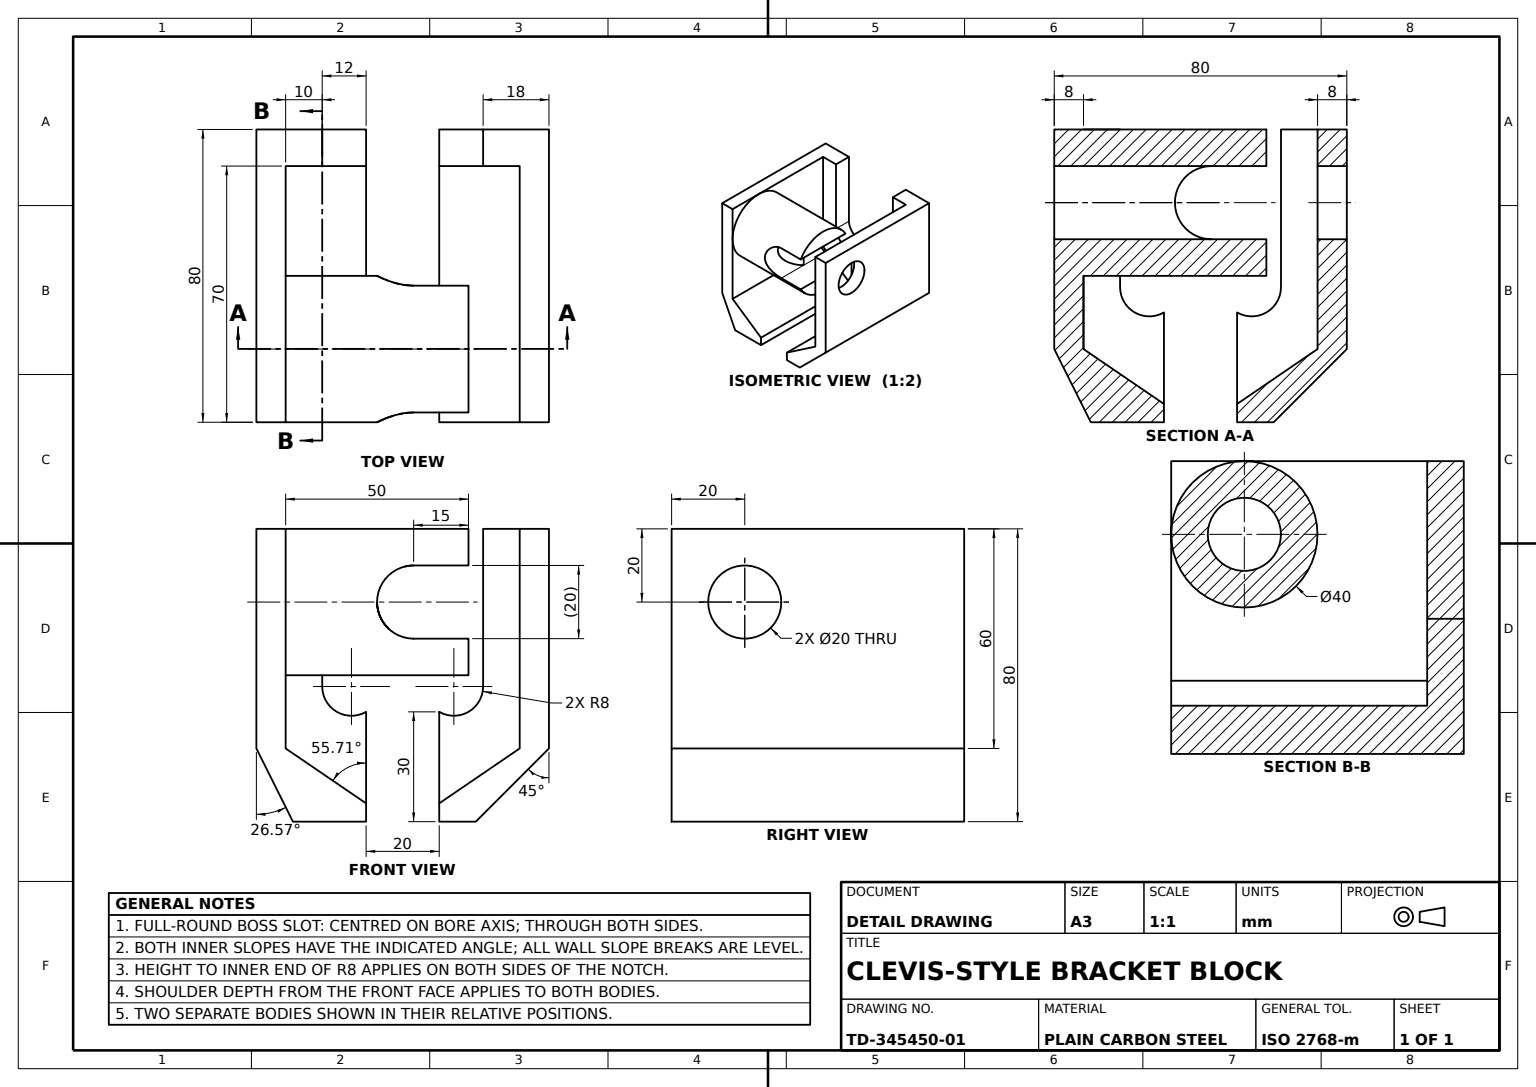
SolidWorks part; units mm, degrees
material "Plain Carbon Steel"
ref_plane "Front Plane" through (0, 0, 0) normal (0, 0, 1) x (1, 0, 0)
ref_plane "Top Plane" through (0, 0, 0) normal (0, 1, 0) x (1, 0, 0)
ref_plane "Right Plane" through (0, 0, 0) normal (1, 0, 0) x (0, 0, -1)
sketch "Clevis Body Profile Sketch" plane through (0, 0, 0) normal (1, 0, 0) x (0, 0, -1)
  line L7 (0, 0) -> (20, 0)
  line L11 (30, 20) -> (20, 0)
  line L12 (0, 0) -> (0, 30)
  line L13 (30, 20) -> (30, 80)
  line L14 (30, 80) -> (12, 80)
  line L15 (12, 80) -> (12, 36.9282)
  arc A1 (0, 30) -> (12, 36.9282) centre (4, 36.9282) ccw
  dimension "D8" = 17.8885
  dimension "D3" = 16
  dimension "D2" = 12
  dimension "D4" = 30
  dimension "D5" = 30
  dimension "D6" = 80
  dimension "D7" = 20
extrude "Clevis Body" add sketch "Clevis Body Profile Sketch" along normal mid plane 80
sketch "Clevis Slot Sketch" plane through (0, 80, 0) normal (0, 1, 0) x (1, 0, 0)
  line L0 (40, 30) -> (-40, 30)
  line L1 (-40, 30) -> (-40, 12)
  line L2 (-40, 12) -> (30, 12)
  line L3 (40, 12) -> (-40, 12) construction
  line L4 (30, 12) -> (30, 22)
  line L5 (30, 22) -> (40, 22)
  line L6 (40, 30) -> (40, 12) construction
  line L7 (40, 22) -> (40, 30)
  line L8 (30, 22) -> (-40, 22)
  line L9 (-40, 22) -> (-40, 12)
  line L10 (40, 22) -> (40, 12)
  line L11 (40, 12) -> (30, 12)
  line L12 (-40, 12) -> (-40, 0)
  line L13 (-40, 0) -> (30, 0)
  line L14 (40, 0) -> (-40, 0) construction
  line L15 (30, 0) -> (30, 12)
  line L16 (-40, 30) -> (-40, 12) construction
  line M8 (-40, 12) -> (40, 12)
  dimension "D1" = 70
extrude "Clevis Slot Cut" cut sketch "Clevis Slot Sketch" against normal blind 60 contours L4 L8 L1 M8 | L13 L15 L12 M8
sketch "Clevis Relief Sketch" plane through (-40, 0, 0) normal (-1, 0, 0) x (0, 0, 1)
  line L0 (0, 0) -> (0, 5)
  line L1 (0, 20) -> (0, 0) construction
  line L2 (0, 5) -> (-22, 20)
  line L3 (-22, 20) -> (0, 20)
  line L4 (0, 20) -> (0, 5)
  line L5 (-22, 20) -> (0, 20) construction
  line M1 (0, 20) -> (-22, 20)
  line M7 (0, 0) -> (0, 20)
  dimension "D1" = 15
extrude "Clevis Relief Cut" cut sketch "Clevis Relief Sketch" against normal blind 70 contours L2 M7 M1
ref_plane "Plane1" through (0, 0, 10) normal (0, 0, 1) x (1, 0, 0)
ref_plane "Plane2" through (40, 0, 0) normal (1, 0, 0) x (0, 0, -1)
sketch "Bracket Body Profile Sketch" plane through (40, 0, 0) normal (1, 0, 0) x (0, 0, -1)
  line L0 (0, 0) -> (-30, 0)
  line L3 (-50, 20) -> (-30, 0)
  line L4 (-50, 20) -> (-50, 80)
  line L5 (-50, 80) -> (-32, 80)
  line L6 (0, 0) -> (-20, 0)
  line L7 (-20, 0) -> (-20, 30)
  line L8 (-32, 80) -> (-32, 36.9282)
  line L9 (0, 30) -> (0, 0) construction
  arc A0 (-32, 36.9282) -> (-20, 30) centre (-24, 36.9282) ccw
  circle A1 centre (0, 0) radius 1
  dimension "D3" = 8
  dimension "D1" = 20
  dimension "D2" = 60
  dimension "D4" = 50
  dimension "D5" = 18
  dimension "D6" = 80
  dimension "D7" = 20
  dimension "D8" = 30
extrude "Bracket Body" add sketch "Bracket Body Profile Sketch" against normal blind 80 separate body contours A0 L8 L5 L4 L3 L0 L7
sketch "Bracket Pocket Sketch" plane through (0, 80, 0) normal (0, 1, 0) x (1, 0, 0)
  line L0 (30, -12.8537) -> (30, -32)
  line L1 (-40, -32) -> (40, -32) construction
  line L3 (-40, -50) -> (-40, -32) construction
  line L4 (-40, -32) -> (-40, -42)
  line L5 (-40, -42) -> (30, -42)
  line L6 (30, -42) -> (30, -32)
  line L7 (-40, -32) -> (-40, -12.8537)
  line L8 (-40, -12.8537) -> (30, -12.8537)
  line L9 (40, -50) -> (40, -32) construction
  dimension "D1" = 10
  dimension "D2" = 19.1463
  dimension "D3" = 10
extrude "Bracket Pocket Cut" cut sketch "Bracket Pocket Sketch" against normal blind 60
sketch "Bracket Notch Sketch" plane through (-40, 0, 0) normal (-1, 0, 0) x (0, 0, 1)
  line L0 (50, 80) -> (42, 80) construction
  line L1 (20, 0) -> (20, 20) construction
  line L2 (20, 5) -> (42, 20)
  line L3 (42, 20) -> (20, 20)
  line L4 (20, 20) -> (20, 5)
  dimension "D1" = 75
extrude "Bracket Notch Cut" cut sketch "Bracket Notch Sketch" against normal blind 70
sketch "Pin Boss Sketch" plane through (0, 0, -22) normal (0, 0, 1) x (1, 0, 0)
  line L0 (-40, 80) -> (-20, 80)
  line L1 (-40, 80) -> (40, 80) construction
  circle A0 centre (-20, 60) radius 20
  dimension "D1" = 40
extrude "Pin Boss" add sketch "Pin Boss Sketch" along normal blind 50 contours A0
sketch "Pin Boss Trim Sketch" plane through (0, 0, 0) normal (1, 0, 0) x (0, 0, -1)
  line L2 (-28, 80) -> (-28, 40) construction
  line L3 (-13, 70) -> (-28, 70)
  line L4 (-28, 70) -> (-28, 50)
  line L5 (-28, 50) -> (-13, 50)
  arc A0 (-13, 50) -> (-13, 70) centre (-13, 60) ccw
  dimension "D1" = 10
  dimension "D2" = 15
  dimension "D3" = 60
extrude "Pin Boss Trim Cut" cut sketch "Pin Boss Trim Sketch" against normal blind 50
sketch "Pin Hole Sketch" plane through (0, 0, -30) normal (0, 0, -1) x (-1, 0, 0)
  line L0 (40, 20) -> (40, 80) construction
  line L1 (-40, 80) -> (40, 80) construction
  circle A0 centre (20, 60) radius 10
  dimension "D1" = 20
  dimension "D2" = 20
  dimension "D3" = 20
extrude "Pin Hole Through" cut sketch "Pin Hole Sketch" against normal blind 88
